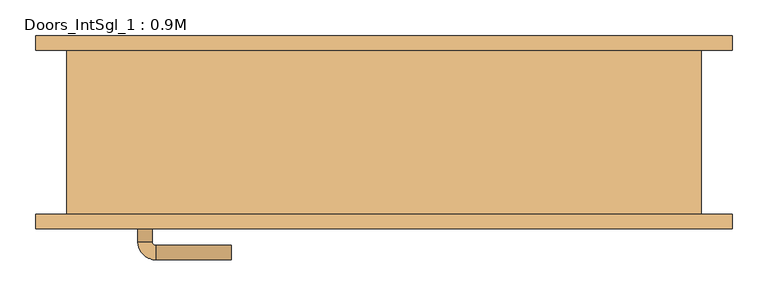
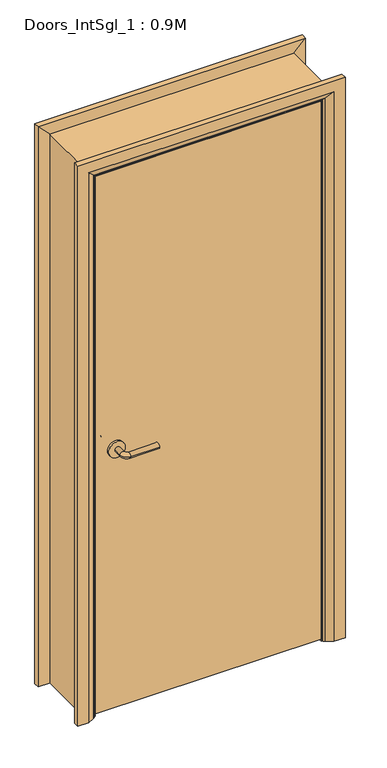
"""IFC4 building model written with IfcOpenShell, lengths in millimetres: door geometry, Doors_IntSgl_1 : 0.9M."""

from ifc_helpers import new_model, si_unit, point, frame, frame_2d, origin, place, context, project, spatial, polyline, circle_curve, ellipse_curve, trimmed, segment, composite_curve, outline, extrude, faceted_brep, source, transform, mapped, element, save
from ifc_brep_helpers import plane_surface, cylinder_surface, revolved_surface, advanced_brep


def doors_intsgl_1_0_9m_9bbf83a0(model_context):
    return source(origin(), model_context, "Body", "SolidModel", [
        advanced_brep(
        [(-343.0, -68.3, 1000.0), (-323.0, -68.3, 1000.0), (-343.0, -38.3, 1000.0), (-323.0, -38.3, 1000.0), (-318.0, -33.3, 1000.0), (-318.0, -13.3, 1000.0), (-213.0, -13.3, 1000.0), (-213.0, -33.3, 1000.0)],
        [
            (0, 1, circle_curve(frame((-333.0, -68.3, 1000.0), z_axis=(0.0, -1.0, 0.0), x_axis=(1.0, 0.0, 0.0)), 10.0)),
            (1, 0, circle_curve(frame((-333.0, -68.3, 1000.0), z_axis=(0.0, -1.0, 0.0), x_axis=(1.0, 0.0, 0.0)), 10.0)),
            (0, 2),
            (2, 3, circle_curve(frame((-333.0, -38.3, 1000.0), z_axis=(0.0, -1.0, 0.0), x_axis=(1.0, 0.0, 0.0)), 10.0)),
            (3, 1),
            (3, 2, circle_curve(frame((-333.0, -38.3, 1000.0), z_axis=(0.0, -1.0, 0.0), x_axis=(1.0, 0.0, 0.0)), 10.0)),
            (4, 3, circle_curve(frame((-318.0, -38.3, 1000.0), z_axis=(0.0, 0.0, 1.0), x_axis=(-1.0, 0.0, 0.0)), 5.0)),
            (2, 5, circle_curve(frame((-318.0, -38.3, 1000.0), z_axis=(0.0, 0.0, -1.0), x_axis=(-1.0, 0.0, 0.0)), 25.0)),
            (5, 4, circle_curve(frame((-318.0, -23.3, 1000.0), z_axis=(-1.0, 0.0, 0.0), x_axis=(0.0, -1.0, 0.0)), 10.0)),
            (4, 5, circle_curve(frame((-318.0, -23.3, 1000.0), z_axis=(-1.0, 0.0, 0.0), x_axis=(0.0, -1.0, 0.0)), 10.0)),
            (6, 7, circle_curve(frame((-213.0, -23.3, 1000.0), z_axis=(1.0, 0.0, 0.0), x_axis=(0.0, -1.0, 0.0)), 10.0)),
            (7, 6, circle_curve(frame((-213.0, -23.3, 1000.0), z_axis=(1.0, 0.0, 0.0), x_axis=(0.0, -1.0, 0.0)), 10.0)),
            (5, 6),
            (7, 4),
        ],
        [
            plane_surface(frame((-333.0, -68.3, 1000.0), z_axis=(0.0, -1.0, 0.0), x_axis=(0.0, 0.0, 1.0))),
            cylinder_surface(frame((-333.0, -68.3, 1000.0), z_axis=(0.0, -1.0, 0.0), x_axis=(1.0, 0.0, 0.0)), 10.0),
            revolved_surface(trimmed(ellipse_curve(frame((-333.0, -38.3, 1000.0), z_axis=(0.0, -1.0, 0.0), x_axis=(1.0, 0.0, 0.0)), 10.0, 10.0), [point((-343.0, -38.3, 1000.0))], [point((-323.0, -38.3, 1000.0))], True, "CARTESIAN"), (-318.0, -38.3, 1000.0), (0.0, 0.0, -1.0)),
            revolved_surface(trimmed(ellipse_curve(frame((-333.0, -38.3, 1000.0), z_axis=(0.0, -1.0, 0.0), x_axis=(1.0, 0.0, 0.0)), 10.0, 10.0), [point((-323.0, -38.3, 1000.0))], [point((-343.0, -38.3, 1000.0))], True, "CARTESIAN"), (-318.0, -38.3, 1000.0), (0.0, 0.0, -1.0)),
            plane_surface(frame((-213.0, -23.3, 1000.0), z_axis=(1.0, 0.0, 0.0), x_axis=(0.0, 0.0, 1.0))),
            cylinder_surface(frame((-318.0, -23.3, 1000.0), z_axis=(-1.0, 0.0, 0.0), x_axis=(0.0, -1.0, 0.0)), 10.0),
        ],
        [
            (0, [[1, 2]]),
            (1, [[-1, 3, 4, 5]]),
            (1, [[-2, -5, 6, -3]]),
            (2, [[7, -4, 8, 9]]),
            (3, [[-8, -6, -7, 10]]),
            (4, [[11, 12]]),
            (5, [[-9, 13, -12, 14]]),
            (5, [[-10, -14, -11, -13]]),
        ],
    ),
        extrude(outline(composite_curve([segment(trimmed(circle_curve(frame_2d((1000.0, -335.5)), 30.0), [point((1000.0, -365.5))], [point((1000.0, -305.5))], False, "CARTESIAN"), True, "CONTINUOUS"), segment(trimmed(circle_curve(frame_2d((1000.0, -335.5)), 30.0), [point((1000.0, -305.5))], [point((1000.0, -365.5))], False, "CARTESIAN"), True, "CONTINUOUS")], self_intersect=False)), frame((0.0, -76.3, 0.0), z_axis=(0.0, 1.0, 0.0), x_axis=(0.0, 0.0, 1.0)), (0.0, 0.0, 1.0), 8.0),
        advanced_brep(
        [(-343.0, -122.3, 1000.0), (-323.0, -122.3, 1000.0), (-323.0, -152.3, 1000.0), (-343.0, -152.3, 1000.0), (-318.0, -157.3, 1000.0), (-318.0, -177.3, 1000.0), (-213.0, -177.3, 1000.0), (-213.0, -157.3, 1000.0)],
        [
            (0, 1, circle_curve(frame((-333.0, -122.3, 1000.0), z_axis=(0.0, 1.0, 0.0), x_axis=(1.0, 0.0, 0.0)), 10.0)),
            (1, 0, circle_curve(frame((-333.0, -122.3, 1000.0), z_axis=(0.0, 1.0, 0.0), x_axis=(1.0, 0.0, 0.0)), 10.0)),
            (1, 2),
            (2, 3, circle_curve(frame((-333.0, -152.3, 1000.0), z_axis=(0.0, 1.0, 0.0), x_axis=(1.0, 0.0, 0.0)), 10.0)),
            (3, 0),
            (3, 2, circle_curve(frame((-333.0, -152.3, 1000.0), z_axis=(0.0, 1.0, 0.0), x_axis=(1.0, 0.0, 0.0)), 10.0)),
            (4, 5, circle_curve(frame((-318.0, -167.3, 1000.0), z_axis=(-1.0, 0.0, 0.0), x_axis=(0.0, 1.0, 0.0)), 10.0)),
            (5, 3, circle_curve(frame((-318.0, -152.3, 1000.0), z_axis=(0.0, 0.0, -1.0), x_axis=(-1.0, 0.0, 0.0)), 25.0)),
            (2, 4, circle_curve(frame((-318.0, -152.3, 1000.0), z_axis=(0.0, 0.0, 1.0), x_axis=(-1.0, 0.0, 0.0)), 5.0)),
            (5, 4, circle_curve(frame((-318.0, -167.3, 1000.0), z_axis=(-1.0, 0.0, 0.0), x_axis=(0.0, 1.0, 0.0)), 10.0)),
            (6, 7, circle_curve(frame((-213.0, -167.3, 1000.0), z_axis=(1.0, 0.0, 0.0), x_axis=(0.0, 1.0, 0.0)), 10.0)),
            (7, 6, circle_curve(frame((-213.0, -167.3, 1000.0), z_axis=(1.0, 0.0, 0.0), x_axis=(0.0, 1.0, 0.0)), 10.0)),
            (4, 7),
            (6, 5),
        ],
        [
            plane_surface(frame((-333.0, -122.3, 1000.0), z_axis=(0.0, 1.0, 0.0), x_axis=(0.0, 0.0, 1.0))),
            cylinder_surface(frame((-333.0, -122.3, 1000.0), z_axis=(0.0, 1.0, 0.0), x_axis=(1.0, 0.0, 0.0)), 10.0),
            revolved_surface(trimmed(ellipse_curve(frame((-333.0, -152.3, 1000.0), z_axis=(0.0, -1.0, 0.0), x_axis=(1.0, 0.0, 0.0)), 10.0, 10.0), [point((-343.0, -152.3, 1000.0))], [point((-323.0, -152.3, 1000.0))], True, "CARTESIAN"), (-318.0, -152.3, 1000.0), (0.0, 0.0, -1.0)),
            revolved_surface(trimmed(ellipse_curve(frame((-333.0, -152.3, 1000.0), z_axis=(0.0, -1.0, 0.0), x_axis=(1.0, 0.0, 0.0)), 10.0, 10.0), [point((-323.0, -152.3, 1000.0))], [point((-343.0, -152.3, 1000.0))], True, "CARTESIAN"), (-318.0, -152.3, 1000.0), (0.0, 0.0, -1.0)),
            plane_surface(frame((-213.0, -167.3, 1000.0), z_axis=(1.0, 0.0, 0.0), x_axis=(0.0, 0.0, 1.0))),
            cylinder_surface(frame((-318.0, -167.3, 1000.0), z_axis=(-1.0, 0.0, 0.0), x_axis=(0.0, 1.0, 0.0)), 10.0),
        ],
        [
            (0, [[1, 2]]),
            (1, [[3, 4, 5, -2]]),
            (1, [[-5, 6, -3, -1]]),
            (2, [[7, 8, -4, 9]]),
            (3, [[10, -9, -6, -8]]),
            (4, [[11, 12]]),
            (5, [[13, -11, 14, -7]]),
            (5, [[-14, -12, -13, -10]]),
        ],
    ),
        extrude(outline(composite_curve([segment(trimmed(circle_curve(frame_2d((1000.0, -335.5)), 30.0), [point((1000.0, -365.5))], [point((1000.0, -305.5))], False, "CARTESIAN"), True, "CONTINUOUS"), segment(trimmed(circle_curve(frame_2d((1000.0, -335.5)), 30.0), [point((1000.0, -305.5))], [point((1000.0, -365.5))], False, "CARTESIAN"), True, "CONTINUOUS")], self_intersect=False)), frame((0.0, -122.3, 0.0), z_axis=(0.0, 1.0, 0.0), x_axis=(0.0, 0.0, 1.0)), (0.0, 0.0, 1.0), 8.0),
        extrude(outline(polyline([(408.0, -76.3), (408.0, -114.3), (-408.0, -114.3), (-408.0, -76.3), (408.0, -76.3)])), frame((0.0, 0.0, 8.0), z_axis=(0.0, 0.0, 1.0), x_axis=(1.0, 0.0, 0.0)), (0.0, 0.0, 1.0), 2060.0),
        faceted_brep([(-410.0, -114.3, 0.0), (-442.0, -114.3, 0.0), (-442.0, 114.3, 0.0), (-410.0, 114.3, 0.0), (-410.0, 114.3, 2070.0), (-410.0, -114.3, 2070.0), (-442.0, 114.3, 2102.0), (-442.0, -114.3, 2102.0), (410.0, -114.3, 0.0), (410.0, 114.3, 0.0), (442.0, 114.3, 0.0), (442.0, -114.3, 0.0), (410.0, -114.3, 2070.0), (442.0, -114.3, 2102.0), (442.0, 114.3, 2102.0), (410.0, 114.3, 2070.0)], [[[0, 1, 2, 3]], [[3, 4, 5, 0]], [[2, 6, 4, 3]], [[1, 7, 6, 2]], [[0, 5, 7, 1]], [[8, 9, 10, 11]], [[12, 8, 11, 13]], [[13, 11, 10, 14]], [[14, 10, 9, 15]], [[15, 9, 8, 12]], [[4, 15, 12, 5]], [[6, 14, 15, 4]], [[7, 13, 14, 6]], [[5, 12, 13, 7]]]),
        advanced_brep(
        [(-485.0, 134.3, 0.0), (-445.0, 134.3, 0.0), (-419.0, 120.3, 0.0), (-415.0, 114.3, 0.0), (-485.0, 114.3, 0.0), (-485.0, 114.3, 2145.0), (-485.0, 134.3, 2145.0), (-415.0, 114.3, 2075.0), (-419.0, 120.3, 2079.0), (-445.0, 134.3, 2105.0), (485.0, 134.3, 0.0), (485.0, 114.3, 0.0), (415.0, 114.3, 0.0), (419.0, 120.3, 0.0), (445.0, 134.3, 0.0), (485.0, 134.3, 2145.0), (445.0, 134.3, 2105.0), (419.0, 120.3, 2079.0), (415.0, 114.3, 2075.0), (485.0, 114.3, 2145.0)],
        [
            (0, 1),
            (1, 2),
            (2, 3, circle_curve(frame((-423.0, 113.3, 0.0), z_axis=(0.0, 0.0, -1.0), x_axis=(-1.0, 0.0, 0.0)), 8.0622577)),
            (3, 4),
            (4, 0),
            (4, 5),
            (5, 6),
            (6, 0),
            (3, 7),
            (7, 5),
            (2, 8),
            (8, 7, ellipse_curve(frame((-423.0, 113.3, 2083.0), z_axis=(-0.7071067811865475, 0.0, -0.7071067811865475), x_axis=(0.7071067811865474, 0.0, -0.7071067811865476)), 11.4017543, 8.0622577)),
            (1, 9),
            (9, 8),
            (6, 9),
            (10, 11),
            (11, 12),
            (12, 13, circle_curve(frame((423.0, 113.3, 0.0), z_axis=(0.0, 0.0, -1.0), x_axis=(1.0, 0.0, 0.0)), 8.0622577)),
            (13, 14),
            (14, 10),
            (15, 10),
            (14, 16),
            (16, 15),
            (13, 17),
            (17, 16),
            (12, 18),
            (18, 17, ellipse_curve(frame((423.0, 113.3, 2083.0), z_axis=(0.7071067811865475, 0.0, -0.7071067811865475), x_axis=(0.7071067811865474, 0.0, 0.7071067811865476)), 11.4017543, 8.0622577)),
            (11, 19),
            (19, 18),
            (15, 19),
            (5, 19),
            (15, 6),
            (7, 18),
            (8, 17),
            (9, 16),
        ],
        [
            plane_surface(frame((-415.0, 187.1010989, 0.0), z_axis=(0.0, 0.0, -1.0), x_axis=(1.0, 0.0, 0.0))),
            plane_surface(frame((-485.0, 134.3, 0.0), z_axis=(-1.0, 0.0, 0.0), x_axis=(0.0, 0.0, 1.0))),
            plane_surface(frame((-485.0, 114.3, 0.0), z_axis=(0.0, -1.0, 0.0), x_axis=(0.0, 0.0, 1.0))),
            cylinder_surface(frame((-423.0, 113.3, 0.0), z_axis=(0.0, 0.0, -1.0), x_axis=(-1.0, 0.0, 0.0)), 8.0622577),
            plane_surface(frame((-419.0, 120.3, 0.0), z_axis=(0.4740998230350183, 0.8804710999221749, 0.0), x_axis=(0.0, 0.0, 1.0))),
            plane_surface(frame((-445.0, 134.3, 0.0), z_axis=(0.0, 1.0, 0.0), x_axis=(0.0, 0.0, 1.0))),
            plane_surface(frame((415.0, 187.1010989, 0.0), z_axis=(0.0, 0.0, -1.0), x_axis=(-1.0, 0.0, 0.0))),
            plane_surface(frame((445.0, 134.3, 2105.0), z_axis=(0.0, 1.0, 0.0), x_axis=(0.0, 0.0, -1.0))),
            plane_surface(frame((419.0, 120.3, 2079.0), z_axis=(-0.4740998230350183, 0.8804710999221749, 0.0), x_axis=(0.0, 0.0, -1.0))),
            cylinder_surface(frame((423.0, 113.3, 2075.0), z_axis=(0.0, 0.0, 1.0), x_axis=(1.0, 0.0, 0.0)), 8.0622577),
            plane_surface(frame((485.0, 114.3, 2145.0), z_axis=(0.0, -1.0, 0.0), x_axis=(0.0, 0.0, -1.0))),
            plane_surface(frame((485.0, 134.3, 2145.0), z_axis=(1.0, 0.0, 0.0), x_axis=(0.0, 0.0, -1.0))),
            plane_surface(frame((-485.0, 134.3, 2145.0), z_axis=(0.0, 0.0, 1.0), x_axis=(1.0, 0.0, 0.0))),
            plane_surface(frame((-485.0, 114.3, 2145.0), z_axis=(0.0, -1.0, 0.0), x_axis=(1.0, 0.0, 0.0))),
            cylinder_surface(frame((-415.0, 113.3, 2083.0), z_axis=(-1.0, 0.0, 0.0), x_axis=(0.0, 0.0, 1.0)), 8.0622577),
            plane_surface(frame((-419.0, 120.3, 2079.0), z_axis=(0.0, 0.8804710999221749, -0.4740998230350183), x_axis=(1.0, 0.0, 0.0))),
            plane_surface(frame((-445.0, 134.3, 2105.0), z_axis=(0.0, 1.0, 0.0), x_axis=(1.0, 0.0, 0.0))),
        ],
        [
            (0, [[1, 2, 3, 4, 5]]),
            (1, [[6, 7, 8, -5]]),
            (2, [[9, 10, -6, -4]]),
            (3, [[11, 12, -9, -3]]),
            (4, [[13, 14, -11, -2]]),
            (5, [[-8, 15, -13, -1]]),
            (6, [[16, 17, 18, 19, 20]]),
            (7, [[21, -20, 22, 23]]),
            (8, [[-22, -19, 24, 25]]),
            (9, [[-24, -18, 26, 27]]),
            (10, [[-26, -17, 28, 29]]),
            (11, [[-28, -16, -21, 30]]),
            (12, [[31, -30, 32, -7]]),
            (13, [[33, -29, -31, -10]]),
            (14, [[34, -27, -33, -12]]),
            (15, [[35, -25, -34, -14]]),
            (16, [[-32, -23, -35, -15]]),
        ],
    ),
        extrude(outline(polyline([(0.0, -391.0), (2051.0, -391.0), (2051.0, 391.0), (0.0, 391.0), (0.0, 410.0), (2070.0, 410.0), (2070.0, -410.0), (0.0, -410.0), (0.0, -391.0)])), frame((0.0, -74.3, 0.0), z_axis=(0.0, 1.0, 0.0), x_axis=(0.0, 0.0, 1.0)), (0.0, 0.0, 1.0), 32.0),
        advanced_brep(
        [(485.0, -134.3, 0.0), (445.0, -134.3, 0.0), (419.0, -120.3, 0.0), (415.0, -114.3, 0.0), (485.0, -114.3, 0.0), (485.0, -114.3, 2145.0), (485.0, -134.3, 2145.0), (415.0, -114.3, 2075.0), (-415.0, -114.3, 2075.0), (-415.0, -114.3, 0.0), (-485.0, -114.3, 0.0), (-485.0, -114.3, 2145.0), (419.0, -120.3, 2079.0), (445.0, -134.3, 2105.0), (-485.0, -134.3, 2145.0), (-485.0, -134.3, 0.0), (-445.0, -134.3, 0.0), (-445.0, -134.3, 2105.0), (-419.0, -120.3, 0.0), (-419.0, -120.3, 2079.0)],
        [
            (0, 1),
            (1, 2),
            (2, 3, circle_curve(frame((423.0, -113.3, 0.0), z_axis=(0.0, 0.0, -1.0), x_axis=(1.0, 0.0, 0.0)), 8.0622577)),
            (3, 4),
            (4, 0),
            (4, 5),
            (5, 6),
            (6, 0),
            (3, 7),
            (7, 8),
            (8, 9),
            (9, 10),
            (10, 11),
            (11, 5),
            (2, 12),
            (12, 7, ellipse_curve(frame((423.0, -113.3, 2083.0), z_axis=(0.7071067811865475, 0.0, -0.7071067811865475), x_axis=(-0.7071067811865474, 0.0, -0.7071067811865476)), 11.4017543, 8.0622577)),
            (1, 13),
            (13, 12),
            (6, 14),
            (14, 15),
            (15, 16),
            (16, 17),
            (17, 13),
            (10, 15),
            (14, 11),
            (9, 18, circle_curve(frame((-423.0, -113.3, 0.0), z_axis=(0.0, 0.0, -1.0), x_axis=(-1.0, 0.0, 0.0)), 8.0622577)),
            (18, 16),
            (19, 18),
            (8, 19, ellipse_curve(frame((-423.0, -113.3, 2083.0), z_axis=(-0.7071067811865475, 0.0, -0.7071067811865475), x_axis=(-0.7071067811865474, 0.0, 0.7071067811865476)), 11.4017543, 8.0622577)),
            (19, 17),
            (12, 19),
        ],
        [
            plane_surface(frame((415.0, -114.3, 0.0), z_axis=(0.0, 0.0, -1.0), x_axis=(0.0, 1.0, 0.0))),
            plane_surface(frame((485.0, -134.3, 0.0), z_axis=(1.0, 0.0, 0.0), x_axis=(0.0, 0.0, 1.0))),
            plane_surface(frame((485.0, -114.3, 0.0), z_axis=(0.0, 1.0, 0.0), x_axis=(0.0, 0.0, 1.0))),
            cylinder_surface(frame((423.0, -113.3, 0.0), z_axis=(0.0, 0.0, -1.0), x_axis=(1.0, 0.0, 0.0)), 8.0622577),
            plane_surface(frame((419.0, -120.3, 0.0), z_axis=(-0.4740998230350126, -0.880471099922178, 0.0), x_axis=(0.0, 0.0, 1.0))),
            plane_surface(frame((445.0, -134.3, 0.0), z_axis=(0.0, -1.0, 0.0), x_axis=(0.0, 0.0, 1.0))),
            plane_surface(frame((-485.0, -134.3, 2145.0), z_axis=(-1.0, 0.0, 0.0), x_axis=(0.0, 0.0, -1.0))),
            plane_surface(frame((-415.0, -114.3, 0.0), z_axis=(0.0, 0.0, -1.0), x_axis=(0.0, 1.0, 0.0))),
            cylinder_surface(frame((-423.0, -113.3, 2075.0), z_axis=(0.0, 0.0, 1.0), x_axis=(-1.0, 0.0, 0.0)), 8.0622577),
            plane_surface(frame((-419.0, -120.3, 2079.0), z_axis=(0.47409982303501824, -0.8804710999221749, 0.0), x_axis=(0.0, 0.0, -1.0))),
            plane_surface(frame((485.0, -134.3, 2145.0), z_axis=(0.0, 0.0, 1.0), x_axis=(-1.0, 0.0, 0.0))),
            cylinder_surface(frame((415.0, -113.3, 2083.0), z_axis=(1.0, 0.0, 0.0), x_axis=(0.0, 0.0, 1.0)), 8.0622577),
            plane_surface(frame((419.0, -120.3, 2079.0), z_axis=(0.0, -0.8804710999221764, -0.4740998230350154), x_axis=(-1.0, 0.0, 0.0))),
        ],
        [
            (0, [[1, 2, 3, 4, 5]]),
            (1, [[6, 7, 8, -5]]),
            (2, [[9, 10, 11, 12, 13, 14, -6, -4]]),
            (3, [[15, 16, -9, -3]]),
            (4, [[17, 18, -15, -2]]),
            (5, [[-8, 19, 20, 21, 22, 23, -17, -1]]),
            (6, [[-13, 24, -20, 25]]),
            (7, [[-24, -12, 26, 27, -21]]),
            (8, [[28, -26, -11, 29]]),
            (9, [[-22, -27, -28, 30]]),
            (10, [[-14, -25, -19, -7]]),
            (11, [[31, -29, -10, -16]]),
            (12, [[-23, -30, -31, -18]]),
        ],
    ),
    ])


if __name__ == "__main__":
    model = new_model("IFC4")
    model_context = context("Model", 3, world=origin())
    ifc_project = project(units=[si_unit("LENGTHUNIT", "METRE", prefix="MILLI")], contexts=[model_context])
    site = spatial("IfcSite", under=ifc_project)
    building = spatial("IfcBuilding", under=site)
    placement = place(None, origin())
    doors_intsgl_1_0_9m_shape = doors_intsgl_1_0_9m_9bbf83a0(model_context)
    element("IfcDoor", 1, ObjectType="Doors_IntSgl_1 : 0.9M", at=placement, inside=building, context=model_context, shape_type="MappedRepresentation", body=[
        mapped(doors_intsgl_1_0_9m_shape, transform((0.0, 0.0, 0.0), x_axis=(1.0, 0.0, 0.0), y_axis=(0.0, 1.0, 0.0), z_axis=(0.0, 0.0, 1.0))),
    ])
    save(model, "model.ifc")

# Revit data of these elements
# Type "Doors_IntSgl_1 : 0.9M"
#   Type Mark = "57"
#   Type Comments = "Internal Single"
#   Operation = "SingleSwingRight"
#   Construction Type Id = "MDOOR"
#   Manufacturer = "Revit"
#   Keynote = "L20"
#   Description = "Internal Single Door"
#   Analytic Construction = "Metal"
#   UnderCut = 0.008 m
#   Tolerance = 0.002 m
#   Thickness = 0.038 m
#   Structural Tolerance = 0.008 m
#   StopDepth = 0.032 m
#   Stop Thickness = 0.019 m
#   Rough Width = 0.9 m
#   Rough Height = 2.11 m
#   Height to Top Lock Rail = 1.0 m
#   Heat Transfer Coefficient (U) = 3.7021 W/(m²·K)
#   Handle Z Distance = 1.0 m
#   Handle X Distance = 0.075 m
#   Frame Thickness = 0.032 m
#   Door Panel Width = 0.816 m
#   Door Panel Thickness = 0.038 m
#   Door Panel Offset = 0.0 m
#   Height = 2.11 m
#   Width = 0.9 m
#   Door Panel Height = 2.06 m
#   Architrave Setback = 0.005 m
#   Vis - Ironmongery = yes
#   Define Thermal Properties by = 1
#   Material Ironmongery = Door - Handle
#   Material Frame = Door - Frame/Mullion
#   Material Door = Door - Panel
#   Material Architrave = Door - Architrave
#   Visual Light Transmittance = 0
#   Solar Heat Gain Coefficient = 0
#   Function = (empty or 0)
#   Wall Closure = (empty or 0)
# Element 1 (IfcDoor, "Doors_IntSgl_1 : 0.9M")
#   Materials on its faces: "Door - Architrave", "Door - Handle", "Door - Frame/Mullion", "Door - Panel"
# Materials
#   "Door - Handle": colour RGB 0 0 0, transparency 0, Keynote = "P21", Cost = 0
#   "Door - Frame/Mullion": class "Wood", colour RGB 212 179 113, transparency 0, Keynote = "L20", Cost = 0
#   "Door - Panel": class "Wood", colour RGB 210 159 95, transparency 0, Keynote = "L20", Cost = 0
#   "Door - Architrave": class "Wood", colour RGB 154 90 5, transparency 0, Keynote = "P20", Cost = 0
